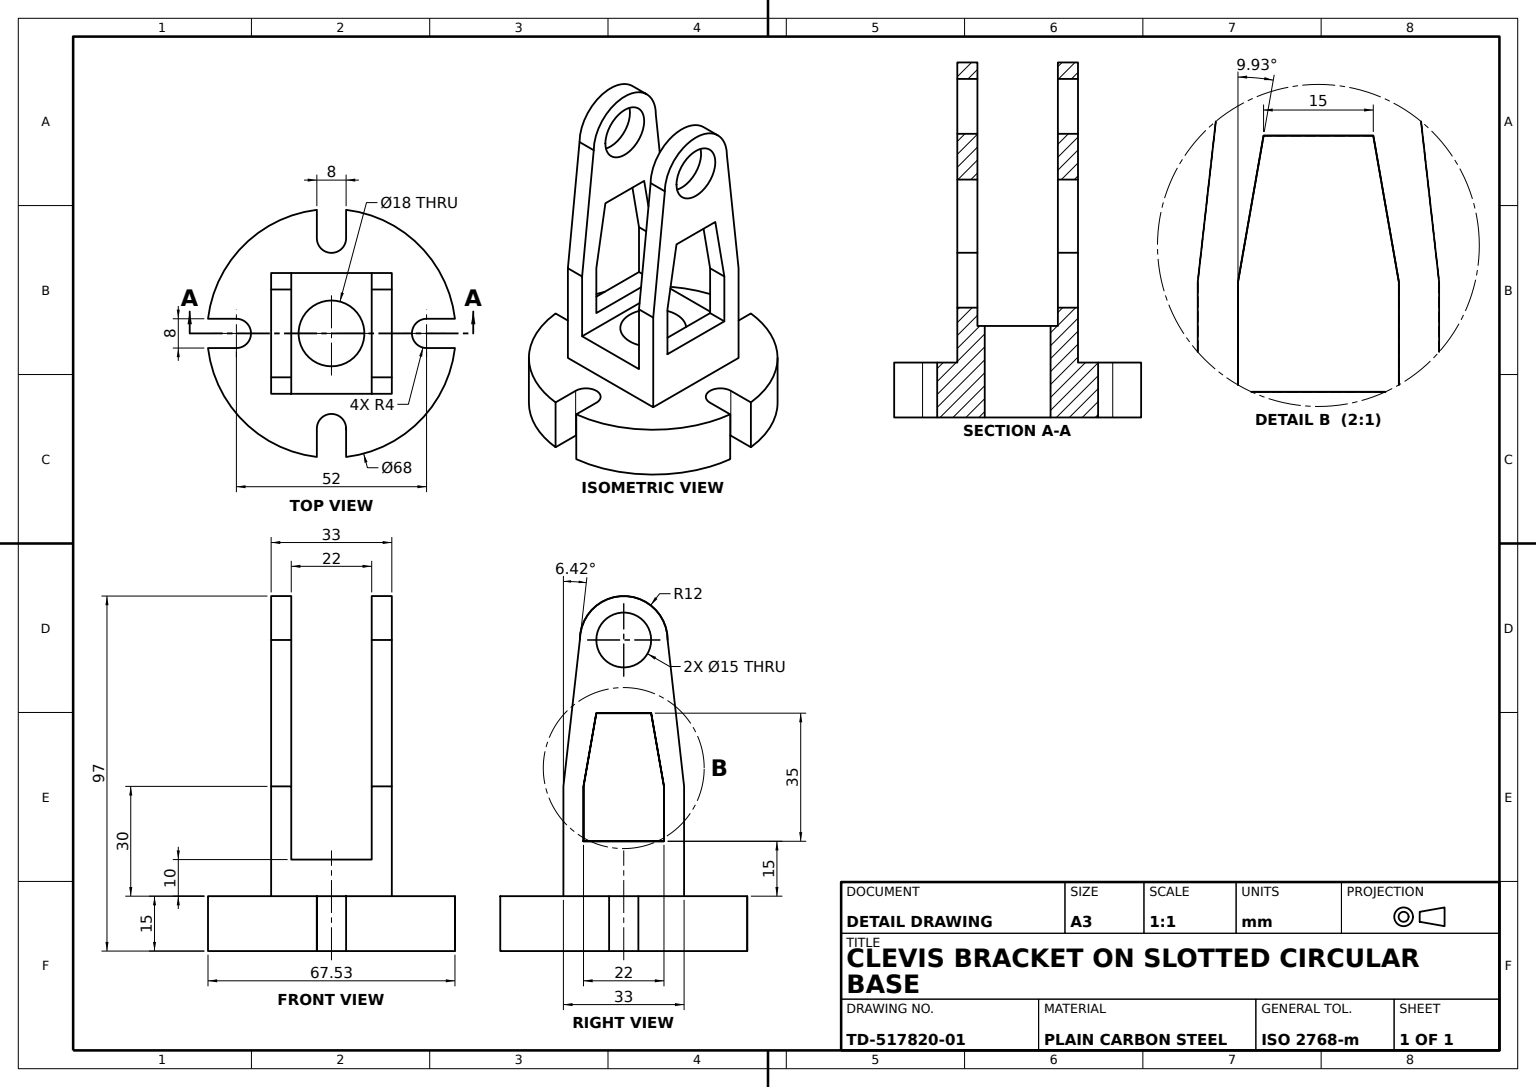
from build123d import *
from build123d.topology import SkipClean

# Parameters (mm, degrees)
BASE_FLANGE_DEPTH       = 15
CENTRE_HOLE_SKETCH_R    = 9
CENTRE_HOLE_18_DEPTH    = 15
LUG_START               = 10
LUG_BASE_PAD_DEPTH      = 10
CLEVIS_LUG_BLOCKS_DEPTH = 70
LUG_PROFILE_CUT_DEPTH   = 54
LUG_EYE_BOSS_DEPTH      = 5.5
LUG_START_2             = -5.5
LUG_WEB_DEPTH           = 5.5


with BuildPart() as part:
    # Base Flange Sketch → Base Flange (new body)
    with BuildSketch(Plane(origin=(0, 0, 0), x_dir=(1, 0, 0), z_dir=(0, 1, 0))):
        with BuildLine():
            ThreePointArc((26, -4), (25.846039759, -3.997035932), (25.692307692, -3.988148122))
            ThreePointArc((25.692307692, -3.988148122), (18.384776311, -18.384776311), (3.988148122, -25.692307692))
            ThreePointArc((3.988148122, -25.692307692), (3.997035932, -25.846039759), (4, -26))
            Line((4, -26), (4, -33.763886032))
            ThreePointArc((4, -33.763886032), (24.04163056, -24.04163056), (33.763886032, -4))
            Line((33.763886032, -4), (26, -4))
        make_face()
        with BuildLine():
            ThreePointArc((25.692307692, 3.988148122), (25.846039759, 3.997035932), (26, 4))
            Line((26, 4), (33.763886032, 4))
            ThreePointArc((33.763886032, 4), (24.04163056, 24.04163056), (4, 33.763886032))
            Line((4, 33.763886032), (4, 26))
            ThreePointArc((4, 26), (3.997035932, 25.846039759), (3.988148122, 25.692307692))
            ThreePointArc((3.988148122, 25.692307692), (18.384776311, 18.384776311), (25.692307692, 3.988148122))
        make_face()
        with BuildLine():
            ThreePointArc((-25.692307692, 3.988148122), (-18.384776311, 18.384776311), (-3.988148122, 25.692307692))
            ThreePointArc((-3.988148122, 25.692307692), (-3.997035932, 25.846039759), (-4, 26))
            Line((-4, 26), (-4, 33.763886032))
            ThreePointArc((-4, 33.763886032), (-24.04163056, 24.04163056), (-33.763886032, 4))
            Line((-33.763886032, 4), (-26, 4))
            ThreePointArc((-26, 4), (-25.846039759, 3.997035932), (-25.692307692, 3.988148122))
        make_face()
        with BuildLine():
            ThreePointArc((-4, -26), (-3.997035932, -25.846039759), (-3.988148122, -25.692307692))
            ThreePointArc((-3.988148122, -25.692307692), (-18.384776311, -18.384776311), (-25.692307692, -3.988148122))
            ThreePointArc((-25.692307692, -3.988148122), (-25.846039759, -3.997035932), (-26, -4))
            Line((-26, -4), (-33.763886032, -4))
            ThreePointArc((-33.763886032, -4), (-24.04163056, -24.04163056), (-4, -33.763886032))
            Line((-4, -33.763886032), (-4, -26))
        make_face()
        with BuildLine():
            ThreePointArc((25.692307692, -3.988148122), (22, 0), (25.692307692, 3.988148122))
            ThreePointArc((25.692307692, 3.988148122), (18.384776311, 18.384776311), (3.988148122, 25.692307692))
            ThreePointArc((3.988148122, 25.692307692), (0, 22), (-3.988148122, 25.692307692))
            ThreePointArc((-3.988148122, 25.692307692), (-18.384776311, 18.384776311), (-25.692307692, 3.988148122))
            ThreePointArc((-25.692307692, 3.988148122), (-22, 0), (-25.692307692, -3.988148122))
            ThreePointArc((-25.692307692, -3.988148122), (-18.384776311, -18.384776311), (-3.988148122, -25.692307692))
            ThreePointArc((-3.988148122, -25.692307692), (0, -22), (3.988148122, -25.692307692))
            ThreePointArc((3.988148122, -25.692307692), (18.384776311, -18.384776311), (25.692307692, -3.988148122))
        make_face()
    extrude(amount=BASE_FLANGE_DEPTH)

    # Centre Hole Sketch → Centre Hole _18 (cut)
    with BuildSketch(Plane(origin=(0, 15, 0), x_dir=(1, 0, 0), z_dir=(0, 1, 0))):
        with Locations(Location((0, 0, 0), (0, 0, 270))):
            Circle(CENTRE_HOLE_SKETCH_R)
    extrude(amount=-CENTRE_HOLE_18_DEPTH, mode=Mode.SUBTRACT)

    # Lug Base Sketch → Lug Base Pad (add)
    with BuildSketch(Plane(origin=(0, 15, 0), x_dir=(1, 0, 0), z_dir=(0, 1, 0)).offset(LUG_START)):
        Polygon((11, -11), (0, -11), (-11, -11), (-11, -16.5), (11, -16.5), align=None)
        Polygon((0, 11), (11, 11), (11, 16.5), (-11, 16.5), (-11, 11), align=None)
        with BuildLine():
            Line((0, -9), (0, -11))
            Line((0, -11), (11, -11))
            Line((11, -11), (11, 11))
            Line((11, 11), (0, 11))
            Line((0, 11), (0, 9))
            ThreePointArc((0, 9), (6.363961031, 6.363961031), (9, 0))
            ThreePointArc((9, 0), (6.363961031, -6.363961031), (0, -9))
        make_face()
        with BuildLine():
            Line((-11, -11), (0, -11))
            Line((0, -11), (0, -9))
            ThreePointArc((0, -9), (-9, 0), (0, 9))
            Line((0, 9), (0, 11))
            Line((0, 11), (-11, 11))
            Line((-11, 11), (-11, -11))
        make_face()
    extrude(amount=-LUG_BASE_PAD_DEPTH)

    # Sketch3_3 → Clevis Lug Blocks (add)
    with BuildSketch(Plane(origin=(0, 15, 0), x_dir=(1, 0, 0), z_dir=(0, 1, 0))):
        Polygon((11, 11), (11, -11), (11, -16.5), (16.5, -16.5), (16.5, 16.5), (11, 16.5), align=None)
        Polygon((-11, -16.5), (-11, -11), (-11, 11), (-11, 16.5), (-16.5, 16.5), (-16.5, -16.5), align=None)
    extrude(amount=CLEVIS_LUG_BLOCKS_DEPTH)

    # Lug Profile Sketch → Lug Profile Cut (cut)
    with BuildSketch(Plane(origin=(16.5, 0, 0), x_dir=(0, 0, -1), z_dir=(1, 0, 0))):
        Polygon((16.5, 85), (12, 85), (16.5, 45), align=None)
        Polygon((-16.5, 45), (-12, 85), (-16.5, 85), align=None)
        Polygon((-11, 30), (-11, 45), (-7.5, 65), (0, 65), (7.5, 65), (11, 45), (11, 30), align=None)
        with BuildLine():
            Line((7.5, 85), (-7.5, 85))
            ThreePointArc((-7.5, 85), (0, 77.5), (7.5, 85))
        make_face()
        with BuildLine():
            ThreePointArc((7.5, 85), (0, 92.5), (-7.5, 85))
            Line((-7.5, 85), (7.5, 85))
        make_face()
    extrude(amount=-LUG_PROFILE_CUT_DEPTH, mode=Mode.SUBTRACT)

    # Sketch6_4 → Lug Eye Boss (add)
    with SkipClean():  # the faces are left unmerged after this step: merging them gives an invalid solid
        with BuildSketch(Plane(origin=(16.5, 0, 0), x_dir=(0, 0, -1), z_dir=(1, 0, 0))):
            with BuildLine():
                Line((-7.5, 85), (-12, 85))
                ThreePointArc((-12, 85), (0, 73), (12, 85))
                Line((12, 85), (7.5, 85))
                ThreePointArc((7.5, 85), (0, 77.5), (-7.5, 85))
            make_face()
            with BuildLine():
                ThreePointArc((12, 85), (0, 97), (-12, 85))
                Line((-12, 85), (-7.5, 85))
                ThreePointArc((-7.5, 85), (0, 92.5), (7.5, 85))
                Line((7.5, 85), (12, 85))
            make_face()
        extrude(amount=-LUG_EYE_BOSS_DEPTH)

    # Lug Web Sketch → Lug Web (add)
    with SkipClean():  # the faces are left unmerged after this step: merging them gives an invalid solid
        with BuildSketch(Plane.ZY.offset(16.5).offset(LUG_START_2)):
            with BuildLine():
                Line((7.5, 85), (12, 85))
                ThreePointArc((12, 85), (0, 97), (-12, 85))
                Line((-12, 85), (-7.5, 85))
                ThreePointArc((-7.5, 85), (0, 92.5), (7.5, 85))
            make_face()
        extrude(amount=LUG_WEB_DEPTH)


solid = part.part
